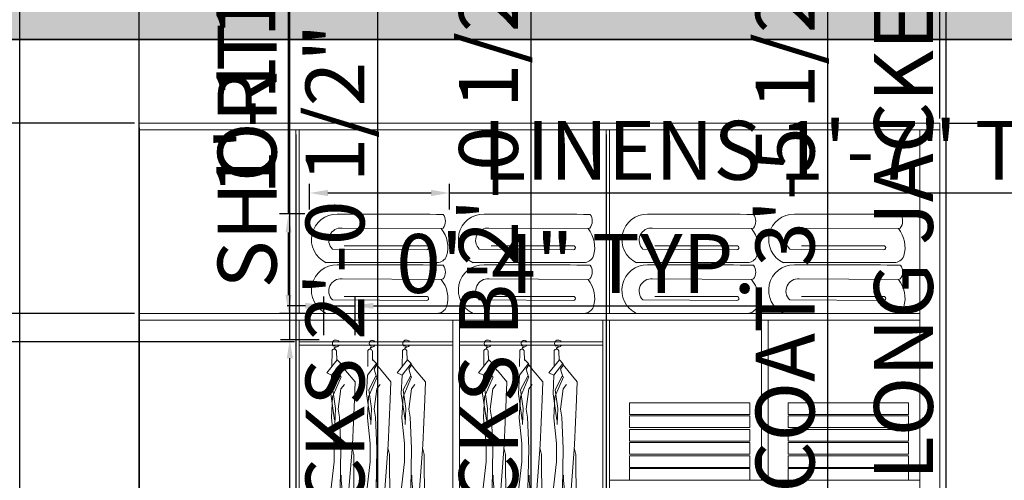
# Model space of a CAD drawing. Units: inches. Extents: x 2257 to 3678, y 834 to 1975.
# Tile 13 of 16: x 3338 to 3471, y 1757 to 1820. Entities that reach past the tile are written whole.
import ezdxf

# ---------------------------------------------------------------- set-up
doc = ezdxf.new("R2010")
doc.units = ezdxf.units.IN
for name, color, linetype, lineweight in [('A-ANNO-DIMS', 2, 'Continuous', 18), ('A-FURN-ELEV', 8, 'Continuous', 13), ('A-SECT', 7, 'Continuous', 35), ('A-SECT-CONC-PATT', 252, 'Continuous', 13)]:
    doc.layers.add(name, color=color, linetype=linetype, lineweight=lineweight)
doc.styles.get("Standard").update_dxf_attribs({"font": 'arial.ttf'})
doc.dimstyles.new('ISO-25', dxfattribs={"dimtxt": 8, "dimasz": 2.5, "dimexe": 1.25, "dimexo": 0.625, "dimtad": 1, "dimdec": 0, "dimlunit": 3, "dimtxsty": 'Standard', "dimcen": 2.5, "dimadec": 0, "dimazin": 0, "dimtfac": 1, "dimtdec": 0, "dimtmove": 0, "dimatfit": 3, "dimfxl": 1, "dimarcsym": 0})

# ---------------------------------------------------------------- blocks, each defined once
blk = doc.blocks.new('WARDROBE-SHELF-LINENS')
for p, q in [((17.6, 11.51), (4.15, 11.59)), ((17.85, 11.57), (17.6, 11.51)), ((2.84, 8.74), (15.61, 8.65)), ((15.54, 9.19), (4.45, 9.19)), ((2, 6.9), (17.02, 6.9)), ((17.6, 4.61), (4.15, 4.7)), ((17.85, 4.68), (17.6, 4.61)), ((2.84, 1.85), (15.61, 1.75)), ((15.54, 2.3), (4.45, 2.3))]:
    blk.add_line(p, q)
for centre, radius, start, end in [((3.45, 10.03), 3.46, 89.4543, 245.1656), ((6.62, -1405.01), 1418.5, 89.54575, 90.12668), ((16.64, 12.53), 1.54, 321.7528, 36.8191), ((4.01, 9.93), 1.67, 85.2319, 225.5868), ((14.47, 8.96), 4.04, 343.4184, 39.2187), ((15.61, 8.93), 0.277, 269.2533, 104.177), ((17.02, 8.31), 1.41, 270, 338.975), ((3.45, 3.14), 3.46, 89.4543, 245.1656), ((6.62, -1411.9), 1418.5, 89.54575, 90.12668), ((16.64, 5.63), 1.54, 321.7528, 36.8191), ((4.01, 3.04), 1.67, 85.2319, 225.5868), ((14.47, 2.06), 4.04, 343.4184, 39.2187), ((15.61, 2.03), 0.277, 269.2533, 104.177), ((17.02, 1.41), 1.41, 270, 338.975)]:
    blk.add_arc(centre, radius, start, end)
blk = doc.blocks.new('WARDROBE-JACKET-SHORT')
for p, q in [((1.8, 28.09), (0.39, 26.33)), ((1.11, 29.37), (1.09, 27.21)), ((1.75, 28.02), (1.71, 29.34)), ((1.8, 28.09), (2.29, 27.6)), ((1.06, 26.01), (2.29, 27.6)), ((2.34, 27.43), (1.96, 26.84)), ((2.29, 25.81), (1.96, 26.84)), ((2.34, 27.43), (2.29, 27.6)), ((2.33, 27.41), (2.93, 26.66)), ((0.39, 26.33), (1.06, 26.01)), ((1.06, 26.01), (0.94, 23.49)), ((2.36, 25.78), (1.19, 23.07)), ((1.23, 24.01), (2.2, 25.86)), ((2.94, 26.66), (4.23, 25.09)), ((1.96, 21.41), (2.32, 24.17)), ((2.32, 24.17), (2.79, 24.73)), ((4.23, 25.09), (4.14, 22.7)), ((0.94, 23.49), (1.46, 19.92)), ((1.19, 23.07), (1.04, 20.22)), ((1.23, 24.01), (1.59, 21.47)), ((1.59, 21.47), (1.5, 19.31)), ((2.14, 20.31), (1.96, 21.41)), ((4.14, 22.7), (3.87, 16.54)), ((1.04, 20.22), (1.4, 16.72)), ((2.32, 16.07), (2.14, 20.31)), ((1.4, 16.72), (1.4, 14.23)), ((2.23, 10.49), (2.32, 16.07)), ((3.87, 16.54), (3.41, 10.49)), ((4.05, 15.25), (3.83, 16.16)), ((4.14, 0), (4.05, 15.25)), ((1.4, 14.23), (0.76, 8.65)), ((2.37, 12.45), (2.37, 11.72)), ((2.37, 11.72), (2.51, 10.41)), ((1.13, 6.07), (2.23, 10.49)), ((3.41, 10.49), (1.94, 2.29)), ((0.76, 8.65), (0.76, 5.61)), ((0.76, 5.61), (0, 0.16)), ((0.4, 3.86), (1.13, 6.07)), ((1.94, 2.29), (0.4, 3.86)), ((1.51, 3.33), (1.49, 1.77)), ((1.47, 1.8), (1.45, 2.53)), ((1.49, 1.77), (1.47, 1.8)), ((0, 0.16), (4.14, 0))]:
    blk.add_line(p, q)
for centre, radius in [((1.45, 30.04), 0.0434), ((1.96, 4.32), 0.103), ((2.03, 4.74), 0.103), ((1.74, 3.32), 0.103), ((1.83, 3.84), 0.103)]:
    blk.add_circle(centre, radius)
for centre, radius, start, end in [((1.64, 30.31), 0.481, 28.9305, 230.329), ((1.4, 29.2), 0.341, 24.2419, 150.7783), ((1.75, 29.53), 0.361, 98.1438, 177.8717), ((1.75, 29.53), 0.315, 98.1438, 177.7449), ((1.64, 30.31), 0.481, 278.1438, 332.6972)]:
    blk.add_arc(centre, radius, start, end)
blk = doc.blocks.new('WARDROBE-JACKET-SHORT-B')
for p, q in [((1.11, 29.37), (1.09, 27.21)), ((1.75, 28.02), (1.72, 29.34)), ((1.8, 28.09), (2.29, 27.6)), ((1.06, 26.01), (2.29, 27.6)), ((2.34, 27.43), (1.96, 26.84)), ((2.29, 25.81), (1.96, 26.84)), ((2.34, 27.43), (2.29, 27.6)), ((2.33, 27.41), (2.94, 26.66)), ((1.06, 26.01), (0.94, 23.49)), ((2.36, 25.78), (1.19, 23.07)), ((1.23, 24.01), (2.2, 25.86)), ((2.94, 26.66), (4.23, 25.09)), ((1.96, 21.41), (2.33, 24.17)), ((2.33, 24.17), (2.79, 24.73)), ((4.23, 25.09), (4.14, 22.7)), ((0.94, 23.49), (1.46, 19.92)), ((1.19, 23.07), (1.04, 20.22)), ((1.23, 24.01), (1.59, 21.47)), ((1.59, 21.47), (1.5, 19.31)), ((2.14, 20.31), (1.96, 21.41)), ((4.14, 22.7), (3.87, 16.54)), ((1.04, 20.22), (1.4, 16.72)), ((2.33, 16.07), (2.14, 20.31)), ((1.4, 16.72), (1.4, 14.23)), ((2.23, 10.49), (2.33, 16.07)), ((3.87, 16.54), (3.41, 10.49)), ((4.05, 15.25), (3.83, 16.16)), ((4.14, 0), (4.05, 15.25)), ((1.4, 14.23), (0.76, 8.65)), ((2.37, 12.45), (2.37, 11.72)), ((2.37, 11.72), (2.52, 10.41)), ((1.13, 6.07), (2.23, 10.49)), ((3.41, 10.49), (1.94, 2.29)), ((0.76, 8.65), (0.76, 5.61)), ((0.76, 5.61), (0, 0.16)), ((0.4, 3.86), (1.13, 6.07)), ((1.94, 2.29), (0.4, 3.86)), ((1.51, 3.33), (1.49, 1.77)), ((1.47, 1.8), (1.45, 2.53)), ((1.49, 1.77), (1.47, 1.8)), ((0, 0.16), (4.14, 0))]:
    blk.add_line(p, q)
for centre, radius in [((1.45, 30.04), 0.0434), ((1.96, 4.32), 0.103), ((2.03, 4.74), 0.103), ((1.74, 3.32), 0.103), ((1.83, 3.84), 0.103)]:
    blk.add_circle(centre, radius)
for centre, radius, start, end in [((1.4, 29.2), 0.341, 24.2419, 150.7783), ((1.67, 30.37), 0.367, 58.8889, 230.4094), ((1.75, 29.53), 0.361, 98.1438, 177.8717), ((1.75, 29.53), 0.315, 98.1438, 177.7449), ((1.64, 30.31), 0.481, 278.1438, 332.6972), ((1.64, 30.31), 0.481, 28.9305, 58.8889)]:
    blk.add_arc(centre, radius, start, end)
blk = doc.blocks.new('*D84')
at = {"layer": 'A-ANNO-DIMS', "color": 0, "lineweight": -2, "transparency": 16777216}
for p, q in [((3377.06, 1793.76), (3377.06, 1797.23)), ((3396.05, 1793.76), (3396.05, 1797.23)), ((3379.56, 1795.98), (3393.55, 1795.98)), ((3396.05, 1795.98), (3491.69, 1795.98))]:
    blk.add_line(p, q, dxfattribs=at)
at = {"layer": 'A-ANNO-DIMS', "color": 0, "transparency": 16777216}
for points in [[(3379.56, 1796.4), (3379.56, 1795.56), (3377.06, 1795.98)], [(3393.55, 1796.4), (3393.55, 1795.56), (3396.05, 1795.98)]]:
    blk.add_solid(points, dxfattribs=at)
at = {"layer": 'Defpoints', "color": 0, "transparency": 16777216}
for p in [(3396.05, 1795.98), (3377.06, 1793.13), (3396.05, 1793.13)]:
    blk.add_point(p, dxfattribs=at)
at = {"layer": 'A-ANNO-DIMS', "color": 0, "transparency": 16777216, "insert": (3445.12, 1800.74), "char_height": 8, "attachment_point": 5}
blk.add_mtext('LINENS 1\'-7" TYP.', dxfattribs=at)
blk = doc.blocks.new('*D85')
at = {"layer": 'A-ANNO-DIMS', "color": 0, "lineweight": -2, "transparency": 16777216}
for p, q in [((3374.21, 1793.13), (3374.21, 1863.53)), ((3376.43, 1793.13), (3372.96, 1793.13)), ((3374.21, 1782.13), (3374.21, 1790.63)), ((3376.43, 1779.63), (3372.96, 1779.63))]:
    blk.add_line(p, q, dxfattribs=at)
at = {"layer": 'A-ANNO-DIMS', "color": 0, "transparency": 16777216}
for points in [[(3373.79, 1790.63), (3374.62, 1790.63), (3374.21, 1793.13)], [(3373.79, 1782.13), (3374.62, 1782.13), (3374.21, 1779.63)]]:
    blk.add_solid(points, dxfattribs=at)
at = {"layer": 'Defpoints', "color": 0, "transparency": 16777216}
for p in [(3374.21, 1793.13), (3377.06, 1793.13), (3377.06, 1779.63)]:
    blk.add_point(p, dxfattribs=at)
at = {"layer": 'A-ANNO-DIMS', "color": 0, "transparency": 16777216, "insert": (3369.44, 1829.58), "char_height": 8, "attachment_point": 5, "rotation": 90}
blk.add_mtext('1\'-1 1/2" TYP.', dxfattribs=at)
blk = doc.blocks.new('*D86')
at = {"layer": 'A-ANNO-DIMS', "color": 0, "lineweight": -2, "transparency": 16777216}
for p, q in [((3374.38, 1776.04), (3374.38, 1916.69)), ((3378.38, 1776.04), (3373.13, 1776.04)), ((3374.38, 1747.73), (3374.38, 1773.54)), ((3378.38, 1745.23), (3373.13, 1745.23))]:
    blk.add_line(p, q, dxfattribs=at)
at = {"layer": 'A-ANNO-DIMS', "color": 0, "transparency": 16777216}
for points in [[(3373.96, 1773.54), (3374.8, 1773.54), (3374.38, 1776.04)], [(3373.96, 1747.73), (3374.8, 1747.73), (3374.38, 1745.23)]]:
    blk.add_solid(points, dxfattribs=at)
at = {"layer": 'Defpoints', "color": 0, "transparency": 16777216}
for p in [(3374.38, 1776.04), (3379, 1776.04), (3379, 1745.23)]:
    blk.add_point(p, dxfattribs=at)
at = {"layer": 'A-ANNO-DIMS', "color": 0, "transparency": 16777216, "insert": (3369.62, 1847.62), "char_height": 8, "attachment_point": 5, "rotation": 90}
blk.add_mtext('SHORT JACKET 2\'-7" TYP.', dxfattribs=at)
blk = doc.blocks.new('*D87')
at = {"layer": 'A-ANNO-DIMS', "color": 0, "lineweight": -2, "transparency": 16777216}
for p, q in [((3379, 1776.67), (3379, 1781.91)), ((3383.24, 1776.67), (3383.24, 1781.91)), ((3376.5, 1780.66), (3374, 1780.66)), ((3379, 1780.66), (3383.24, 1780.66)), ((3385.74, 1780.66), (3438.25, 1780.66))]:
    blk.add_line(p, q, dxfattribs=at)
at = {"layer": 'A-ANNO-DIMS', "color": 0, "transparency": 16777216}
for points in [[(3376.5, 1781.08), (3376.5, 1780.25), (3379, 1780.66)], [(3385.74, 1781.08), (3385.74, 1780.25), (3383.24, 1780.66)]]:
    blk.add_solid(points, dxfattribs=at)
at = {"layer": 'Defpoints', "color": 0, "transparency": 16777216}
for p in [(3383.24, 1780.66), (3379, 1776.04), (3383.24, 1776.04)]:
    blk.add_point(p, dxfattribs=at)
at = {"layer": 'A-ANNO-DIMS', "color": 0, "transparency": 16777216, "insert": (3413.24, 1785.37), "char_height": 8, "attachment_point": 5}
blk.add_mtext('0\'-4" TYP.', dxfattribs=at)
blk = doc.blocks.new('*D88')
at = {"layer": 'A-ANNO-DIMS', "color": 0, "lineweight": -2, "transparency": 16777216}
for p, q in [((3386.31, 1728.42), (3386.31, 1846.75)), ((3383.26, 1728.42), (3387.56, 1728.42)), ((3386.31, 1706.41), (3386.31, 1725.92)), ((3383.26, 1703.91), (3387.56, 1703.91))]:
    blk.add_line(p, q, dxfattribs=at)
at = {"layer": 'A-ANNO-DIMS', "color": 0, "transparency": 16777216}
for points in [[(3385.89, 1725.92), (3386.72, 1725.92), (3386.31, 1728.42)], [(3385.89, 1706.41), (3386.72, 1706.41), (3386.31, 1703.91)]]:
    blk.add_solid(points, dxfattribs=at)
at = {"layer": 'Defpoints', "color": 0, "transparency": 16777216}
for p in [(3382.63, 1728.42), (3386.31, 1728.42), (3382.63, 1703.91)]:
    blk.add_point(p, dxfattribs=at)
at = {"layer": 'A-ANNO-DIMS', "color": 0, "transparency": 16777216, "insert": (3381.55, 1788.84), "char_height": 8, "attachment_point": 5, "rotation": 90}
blk.add_mtext('SLACKS 2\'-0 1/2" TYP.', dxfattribs=at)
blk = doc.blocks.new('*D90')
at = {"layer": 'A-ANNO-DIMS', "color": 0, "lineweight": -2, "transparency": 16777216}
for p, q in [((3463.51, 1750.62), (3463.51, 1883.51)), ((3457.86, 1750.62), (3464.76, 1750.62)), ((3463.51, 1711.27), (3463.51, 1748.12)), ((3457.86, 1708.77), (3464.76, 1708.77))]:
    blk.add_line(p, q, dxfattribs=at)
at = {"layer": 'A-ANNO-DIMS', "color": 0, "transparency": 16777216}
for points in [[(3463.09, 1748.12), (3463.92, 1748.12), (3463.51, 1750.62)], [(3463.09, 1711.27), (3463.92, 1711.27), (3463.51, 1708.77)]]:
    blk.add_solid(points, dxfattribs=at)
at = {"layer": 'Defpoints', "color": 0, "transparency": 16777216}
for p in [(3457.23, 1750.62), (3463.51, 1750.62), (3457.23, 1708.77)]:
    blk.add_point(p, dxfattribs=at)
at = {"layer": 'A-ANNO-DIMS', "color": 0, "transparency": 16777216, "insert": (3458.74, 1818.32), "char_height": 8, "attachment_point": 5, "rotation": 90}
blk.add_mtext('LONG JACKET 3\'-6" TYP.', dxfattribs=at)
blk = doc.blocks.new('*D92')
at = {"layer": 'A-ANNO-DIMS', "color": 0, "lineweight": -2, "transparency": 16777216}
for p, q in [((3447.43, 1750.59), (3447.43, 1855.81)), ((3441.81, 1750.59), (3448.68, 1750.59)), ((3447.43, 1711.44), (3447.43, 1748.09)), ((3441.81, 1708.94), (3448.68, 1708.94))]:
    blk.add_line(p, q, dxfattribs=at)
at = {"layer": 'A-ANNO-DIMS', "color": 0, "transparency": 16777216}
for points in [[(3447.01, 1748.09), (3447.85, 1748.09), (3447.43, 1750.59)], [(3447.01, 1711.44), (3447.85, 1711.44), (3447.43, 1708.94)]]:
    blk.add_solid(points, dxfattribs=at)
at = {"layer": 'Defpoints', "color": 0, "transparency": 16777216}
for p in [(3441.18, 1750.59), (3447.43, 1750.59), (3441.18, 1708.94)]:
    blk.add_point(p, dxfattribs=at)
at = {"layer": 'A-ANNO-DIMS', "color": 0, "transparency": 16777216, "insert": (3442.66, 1804.45), "char_height": 8, "attachment_point": 5, "rotation": 90}
blk.add_mtext('COAT 3\'-5 1/2" TYP.', dxfattribs=at)
blk = doc.blocks.new('*D94')
at = {"layer": 'A-ANNO-DIMS', "color": 0, "lineweight": -2, "transparency": 16777216}
for p, q in [((3407.15, 1728.42), (3407.15, 1857.31)), ((3410.23, 1728.42), (3405.9, 1728.42)), ((3407.15, 1706.24), (3407.15, 1725.92)), ((3410.23, 1703.74), (3405.9, 1703.74))]:
    blk.add_line(p, q, dxfattribs=at)
at = {"layer": 'A-ANNO-DIMS', "color": 0, "transparency": 16777216}
for points in [[(3406.73, 1725.92), (3407.57, 1725.92), (3407.15, 1728.42)], [(3406.73, 1706.24), (3407.57, 1706.24), (3407.15, 1703.74)]]:
    blk.add_solid(points, dxfattribs=at)
at = {"layer": 'Defpoints', "color": 0, "transparency": 16777216}
for p in [(3407.15, 1728.42), (3410.85, 1728.42), (3410.85, 1703.74)]:
    blk.add_point(p, dxfattribs=at)
at = {"layer": 'A-ANNO-DIMS', "color": 0, "transparency": 16777216, "insert": (3402.39, 1794.12), "char_height": 8, "attachment_point": 5, "rotation": 90}
blk.add_mtext('SLACKS B 2\'-0 1/2" TYP.', dxfattribs=at)
blk = doc.blocks.new('*D138')
at = {"layer": 'A-ANNO-DIMS', "color": 0, "lineweight": -2, "transparency": 16777216}
for p, q in [((3353.91, 1806.08), (3353.91, 1897.74)), ((3462.66, 1806.08), (3462.66, 1897.74)), ((3356.41, 1896.49), (3460.16, 1896.49))]:
    blk.add_line(p, q, dxfattribs=at)
at = {"layer": 'A-ANNO-DIMS', "color": 0, "transparency": 16777216}
for points in [[(3356.41, 1896.91), (3356.41, 1896.07), (3353.91, 1896.49)], [(3460.16, 1896.91), (3460.16, 1896.07), (3462.66, 1896.49)]]:
    blk.add_solid(points, dxfattribs=at)
at = {"layer": 'Defpoints', "color": 0, "transparency": 16777216}
for p in [(3462.66, 1896.49), (3353.91, 1805.46), (3462.66, 1805.46)]:
    blk.add_point(p, dxfattribs=at)
at = {"layer": 'A-ANNO-DIMS', "color": 0, "transparency": 16777216, "insert": (3408.29, 1901.2), "char_height": 8, "attachment_point": 5}
blk.add_mtext('9\'-1"', dxfattribs=at)
blk = doc.blocks.new('*D139')
at = {"layer": 'A-ANNO-DIMS', "color": 0, "lineweight": -2, "transparency": 16777216}
for p, q in [((3463.29, 1805.46), (3573.28, 1805.46)), ((3572.03, 1699.2), (3572.03, 1802.96)), ((3463.29, 1696.7), (3573.28, 1696.7))]:
    blk.add_line(p, q, dxfattribs=at)
at = {"layer": 'A-ANNO-DIMS', "color": 0, "transparency": 16777216}
for points in [[(3571.61, 1802.96), (3572.45, 1802.96), (3572.03, 1805.46)], [(3571.61, 1699.2), (3572.45, 1699.2), (3572.03, 1696.7)]]:
    blk.add_solid(points, dxfattribs=at)
at = {"layer": 'Defpoints', "color": 0, "transparency": 16777216}
for p in [(3462.66, 1805.46), (3572.03, 1805.46), (3462.66, 1696.7)]:
    blk.add_point(p, dxfattribs=at)
at = {"layer": 'A-ANNO-DIMS', "color": 0, "transparency": 16777216, "insert": (3567.32, 1751.08), "char_height": 8, "attachment_point": 5, "rotation": 90}
blk.add_mtext('9\'-1"', dxfattribs=at)
blk = doc.blocks.new('*D140')
at = {"layer": 'A-ANNO-DIMS', "color": 0, "lineweight": -2, "transparency": 16777216}
for p, q in [((3337.7, 1697.47), (3337.7, 1897.74)), ((3353.91, 1697.33), (3353.91, 1897.74)), ((3340.2, 1896.49), (3351.41, 1896.49)), ((3353.91, 1896.49), (3378.17, 1896.49))]:
    blk.add_line(p, q, dxfattribs=at)
at = {"layer": 'A-ANNO-DIMS', "color": 0, "transparency": 16777216}
for points in [[(3340.2, 1896.91), (3340.2, 1896.07), (3337.7, 1896.49)], [(3351.41, 1896.91), (3351.41, 1896.07), (3353.91, 1896.49)]]:
    blk.add_solid(points, dxfattribs=at)
at = {"layer": 'Defpoints', "color": 0, "transparency": 16777216}
for p in [(3353.91, 1896.49), (3337.7, 1696.84), (3353.91, 1696.7)]:
    blk.add_point(p, dxfattribs=at)
at = {"layer": 'A-ANNO-DIMS', "color": 0, "transparency": 16777216, "insert": (3367.29, 1901.13), "char_height": 8, "attachment_point": 5}
blk.add_mtext('1\'-4"', dxfattribs=at)
blk = doc.blocks.new('*D143')
at = {"layer": 'A-ANNO-DIMS', "color": 0, "lineweight": -2, "transparency": 16777216}
for p, q in [((3353.91, 1804.83), (3353.91, 1600.44)), ((3375.21, 1803.92), (3375.21, 1600.44)), ((3356.41, 1601.69), (3372.71, 1601.69)), ((3375.21, 1601.69), (3418.11, 1601.69))]:
    blk.add_line(p, q, dxfattribs=at)
at = {"layer": 'A-ANNO-DIMS', "color": 0, "transparency": 16777216}
for points in [[(3356.41, 1602.1), (3356.41, 1601.27), (3353.91, 1601.69)], [(3372.71, 1602.1), (3372.71, 1601.27), (3375.21, 1601.69)]]:
    blk.add_solid(points, dxfattribs=at)
at = {"layer": 'Defpoints', "color": 0, "transparency": 16777216}
for p in [(3353.91, 1805.46), (3375.21, 1804.55), (3375.21, 1601.69)]:
    blk.add_point(p, dxfattribs=at)
at = {"layer": 'A-ANNO-DIMS', "color": 0, "transparency": 16777216, "insert": (3397.91, 1606.45), "char_height": 8, "attachment_point": 5}
blk.add_mtext('1\'-9 1/2"', dxfattribs=at)
blk = doc.blocks.new('*D144')
at = {"layer": 'A-ANNO-DIMS', "color": 0, "lineweight": -2, "transparency": 16777216}
for p, q in [((3375.21, 1803.92), (3375.21, 1600.44)), ((3417.35, 1803.92), (3417.35, 1600.44)), ((3377.71, 1601.69), (3414.85, 1601.69))]:
    blk.add_line(p, q, dxfattribs=at)
at = {"layer": 'A-ANNO-DIMS', "color": 0, "transparency": 16777216}
for points in [[(3377.71, 1602.1), (3377.71, 1601.27), (3375.21, 1601.69)], [(3414.85, 1602.1), (3414.85, 1601.27), (3417.35, 1601.69)]]:
    blk.add_solid(points, dxfattribs=at)
at = {"layer": 'Defpoints', "color": 0, "transparency": 16777216}
for p in [(3375.21, 1804.55), (3417.35, 1804.55), (3417.35, 1601.69)]:
    blk.add_point(p, dxfattribs=at)
at = {"layer": 'A-ANNO-DIMS', "color": 0, "transparency": 16777216, "insert": (3396.28, 1606.4), "char_height": 8, "attachment_point": 5}
blk.add_mtext('3\'-6"', dxfattribs=at)
blk = doc.blocks.new('*D145')
at = {"layer": 'A-ANNO-DIMS', "color": 0, "lineweight": -2, "transparency": 16777216}
for p, q in [((3353.28, 1805.46), (2971.8, 1805.46)), ((2973.05, 1782.13), (2973.05, 1802.96)), ((3353.28, 1779.63), (2971.8, 1779.63))]:
    blk.add_line(p, q, dxfattribs=at)
at = {"layer": 'A-ANNO-DIMS', "color": 0, "transparency": 16777216}
for points in [[(2972.63, 1802.96), (2973.47, 1802.96), (2973.05, 1805.46)], [(2972.63, 1782.13), (2973.47, 1782.13), (2973.05, 1779.63)]]:
    blk.add_solid(points, dxfattribs=at)
at = {"layer": 'Defpoints', "color": 0, "transparency": 16777216}
for p in [(2973.05, 1805.46), (3353.91, 1805.46), (3353.91, 1779.63)]:
    blk.add_point(p, dxfattribs=at)
at = {"layer": 'A-ANNO-DIMS', "color": 0, "transparency": 16777216, "insert": (2968.41, 1792.54), "char_height": 8, "attachment_point": 5, "rotation": 90}
blk.add_mtext('2\'-2"', dxfattribs=at)
blk = doc.blocks.new('*D148')
at = {"layer": 'A-ANNO-DIMS', "color": 0, "lineweight": -2, "transparency": 16777216}
for p, q in [((3375.03, 1775.78), (2971.8, 1775.78)), ((2973.05, 1744.52), (2973.05, 1773.28)), ((3375.03, 1742.02), (2971.8, 1742.02))]:
    blk.add_line(p, q, dxfattribs=at)
at = {"layer": 'A-ANNO-DIMS', "color": 0, "transparency": 16777216}
for points in [[(2972.63, 1773.28), (2973.47, 1773.28), (2973.05, 1775.78)], [(2972.63, 1744.52), (2973.47, 1744.52), (2973.05, 1742.02)]]:
    blk.add_solid(points, dxfattribs=at)
at = {"layer": 'Defpoints', "color": 0, "transparency": 16777216}
for p in [(2973.05, 1775.78), (3375.66, 1775.78), (3375.66, 1742.02)]:
    blk.add_point(p, dxfattribs=at)
at = {"layer": 'A-ANNO-DIMS', "color": 0, "transparency": 16777216, "insert": (2968.34, 1758.9), "char_height": 8, "attachment_point": 5, "rotation": 90}
blk.add_mtext('2\'-10"', dxfattribs=at)

msp = doc.modelspace()

# ---------------------------------------------------------------- hatches: boundary and pattern name
at = {"layer": 'A-SECT-CONC-PATT'}
h = msp.add_hatch(dxfattribs=at)
h.set_pattern_fill('AR-CONC', color=256, scale=0.035, style=0)
h.paths.add_polyline_path([(3004.7, 1816.84), (3502.7, 1816.84), (3502.7, 1822.84), (3004.7, 1822.84)])

# ---------------------------------------------------------------- linework, layer by layer
at = {"layer": 'A-FURN-ELEV'}
for p, q in [((3353.91, 1696.7), (3353.91, 1805.46)), ((3462.66, 1805.46), (3353.91, 1805.46)), ((3462.66, 1696.7), (3462.66, 1805.46)), ((3462.66, 1804.55), (3353.91, 1804.55)), ((3375.21, 1779.63), (3375.21, 1804.55)), ((3375.66, 1779.63), (3375.66, 1804.55)), ((3417.35, 1779.63), (3417.35, 1804.55)), ((3417.8, 1779.63), (3417.8, 1804.55)), ((3459.94, 1701.23), (3459.94, 1804.55)), ((3459.94, 1779.63), (3353.91, 1779.63)), ((3459.94, 1778.72), (3353.91, 1778.72)), ((3375.21, 1701.69), (3375.21, 1778.72)), ((3375.66, 1701.69), (3375.66, 1778.72)), ((3396.5, 1742.02), (3396.5, 1778.72)), ((3397.41, 1742.02), (3397.41, 1778.72)), ((3416.89, 1701.69), (3416.89, 1778.72)), ((3417.8, 1701.69), (3417.8, 1778.72)), ((3438.42, 1756.97), (3438.42, 1778.72)), ((3439.33, 1756.97), (3439.33, 1778.72)), ((3417.8, 1756.97), (3459.94, 1756.97))]:
    msp.add_line(p, q, dxfattribs=at)
for points in [[(3396.5, 1775.78), (3375.66, 1775.78)], [(3416.89, 1775.78), (3397.41, 1775.78)], [(3375.66, 1775.3), (3396.5, 1775.3)], [(3397.41, 1775.3), (3416.89, 1775.3)], [(3420.51, 1756.97), (3420.51, 1758.56), (3436.85, 1758.56), (3436.85, 1756.97)], [(3442.03, 1756.97), (3442.03, 1758.56), (3458.37, 1758.56), (3458.37, 1756.97)]]:
    msp.add_lwpolyline(points, dxfattribs=at)
for points in [[(3420.51, 1767.49), (3436.85, 1767.49), (3436.85, 1765.9), (3420.51, 1765.9)], [(3442.03, 1767.49), (3458.37, 1767.49), (3458.37, 1765.9), (3442.03, 1765.9)], [(3420.51, 1765.73), (3436.85, 1765.73), (3436.85, 1764.13), (3420.51, 1764.13)], [(3442.03, 1765.73), (3458.37, 1765.73), (3458.37, 1764.13), (3442.03, 1764.13)], [(3420.51, 1763.86), (3436.85, 1763.86), (3436.85, 1762.27), (3420.51, 1762.27)], [(3442.03, 1763.86), (3458.37, 1763.86), (3458.37, 1762.27), (3442.03, 1762.27)], [(3420.51, 1762.1), (3436.85, 1762.1), (3436.85, 1760.5), (3420.51, 1760.5)], [(3442.03, 1762.1), (3458.37, 1762.1), (3458.37, 1760.5), (3442.03, 1760.5)], [(3420.51, 1760.28), (3436.85, 1760.28), (3436.85, 1758.69), (3420.51, 1758.69)], [(3442.03, 1760.28), (3458.37, 1760.28), (3458.37, 1758.69), (3442.03, 1758.69)]]:
    msp.add_lwpolyline(points, close=True, dxfattribs=at)
at = {"layer": 'A-SECT'}
msp.add_line((3502.7, 1816.84), (3196.31, 1816.84), dxfattribs=at)

# ---------------------------------------------------------------- block references
at = {"layer": 'A-FURN-ELEV'}
for name, p in [('WARDROBE-SHELF-LINENS', (3377.33, 1779.63)), ('WARDROBE-SHELF-LINENS', (3397.27, 1779.63)), ('WARDROBE-SHELF-LINENS', (3419.47, 1779.63)), ('WARDROBE-SHELF-LINENS', (3439.41, 1779.63)), ('WARDROBE-JACKET-SHORT', (3379, 1745.23)), ('WARDROBE-JACKET-SHORT-B', (3383.87, 1745.23)), ('WARDROBE-JACKET-SHORT', (3388.56, 1745.23)), ('WARDROBE-JACKET-SHORT', (3399.62, 1745.23)), ('WARDROBE-JACKET-SHORT-B', (3404.49, 1745.23)), ('WARDROBE-JACKET-SHORT', (3409.18, 1745.23))]:
    msp.add_blockref(name, p, dxfattribs=at)

# ---------------------------------------------------------------- dimensions: what is measured, and where the dimension line sits
at = {"layer": 'A-ANNO-DIMS'}
for base, p1, p2, text, picture, middle in [((3374.38, 1776.04), (3379, 1745.23), (3379, 1776.04), 'SHORT JACKET <> TYP.', '*D86', (3369.62, 1847.62)), ((3463.5083, 1750.6208), (3457.2306, 1708.7697), (3457.2306, 1750.6208), 'LONG JACKET <> TYP.', '*D90', (3458.7414, 1818.3161)), ((3374.21, 1793.13), (3377.06, 1779.63), (3377.06, 1793.13), '<> TYP.', '*D85', (3369.44, 1829.58)), ((3407.15, 1728.42), (3410.85, 1703.74), (3410.85, 1728.42), 'SLACKS B <> TYP.', '*D94', (3402.39, 1794.12)), ((3447.4307, 1750.5944), (3441.1821, 1708.9374), (3441.1821, 1750.5944), 'COAT <> TYP.', '*D92', (3442.6638, 1804.4506)), ((3386.31, 1728.42), (3382.63, 1703.91), (3382.63, 1728.42), 'SLACKS <> TYP.', '*D88', (3381.55, 1788.84))]:
    dim = msp.add_linear_dim(base=base, p1=p1, p2=p2, angle=90, text=text, dimstyle='ISO-25', override={"dimdec": 1, "dimlfac": 1, "dimrnd": 0, "dimzin": 1, "dimdsep": 46, "dimlunit": 4, "dimfrac": 2}, dxfattribs=at)
    dim.commit()
    dim.dimension.update_dxf_attribs({"geometry": picture, "text_midpoint": middle})
for base, p1, p2, picture, middle in [((3353.91, 1896.49), (3337.7, 1696.84), (3353.91, 1696.7), '*D140', (3367.29, 1901.13)), ((3462.662, 1896.4905), (3353.9086, 1805.4561), (3462.662, 1805.4561), '*D138', (3408.2853, 1901.2001)), ((3375.21, 1601.69), (3353.91, 1805.46), (3375.21, 1804.55), '*D143', (3397.91, 1606.45)), ((3417.35, 1601.69), (3375.21, 1804.55), (3417.35, 1804.55), '*D144', (3396.28, 1606.4))]:
    dim = msp.add_linear_dim(base=base, p1=p1, p2=p2, dimstyle='ISO-25', override={"dimdec": 1, "dimlfac": 1, "dimrnd": 0, "dimzin": 1, "dimdsep": 46, "dimlunit": 4, "dimfrac": 2}, dxfattribs=at)
    dim.commit()
    dim.dimension.update_dxf_attribs({"geometry": picture, "text_midpoint": middle})
for base, p1, p2, text, picture, middle in [((3396.05, 1795.98), (3377.06, 1793.13), (3396.05, 1793.13), 'LINENS <> TYP.', '*D84', (3445.12, 1800.74)), ((3383.24, 1780.66), (3379, 1776.04), (3383.24, 1776.04), '<> TYP.', '*D87', (3413.24, 1785.37))]:
    dim = msp.add_linear_dim(base=base, p1=p1, p2=p2, text=text, dimstyle='ISO-25', override={"dimdec": 1, "dimlfac": 1, "dimrnd": 0, "dimzin": 1, "dimdsep": 46, "dimlunit": 4, "dimfrac": 2}, dxfattribs=at)
    dim.commit()
    dim.dimension.update_dxf_attribs({"geometry": picture, "text_midpoint": middle})
for base, p1, p2, picture, middle in [((2973.05, 1805.46), (3353.91, 1779.63), (3353.91, 1805.46), '*D145', (2968.41, 1792.54)), ((3572.03, 1805.46), (3462.66, 1696.7), (3462.66, 1805.46), '*D139', (3567.32, 1751.08)), ((2973.05, 1775.78), (3375.66, 1742.02), (3375.66, 1775.78), '*D148', (2968.34, 1758.9))]:
    dim = msp.add_linear_dim(base=base, p1=p1, p2=p2, angle=90, dimstyle='ISO-25', override={"dimdec": 1, "dimlfac": 1, "dimrnd": 0, "dimzin": 1, "dimdsep": 46, "dimlunit": 4, "dimfrac": 2}, dxfattribs=at)
    dim.commit()
    dim.dimension.update_dxf_attribs({"geometry": picture, "text_midpoint": middle})

doc.saveas('drawing.dxf')
